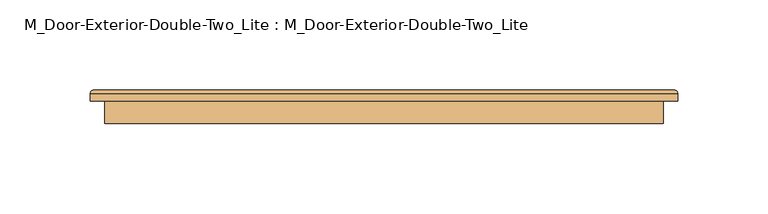
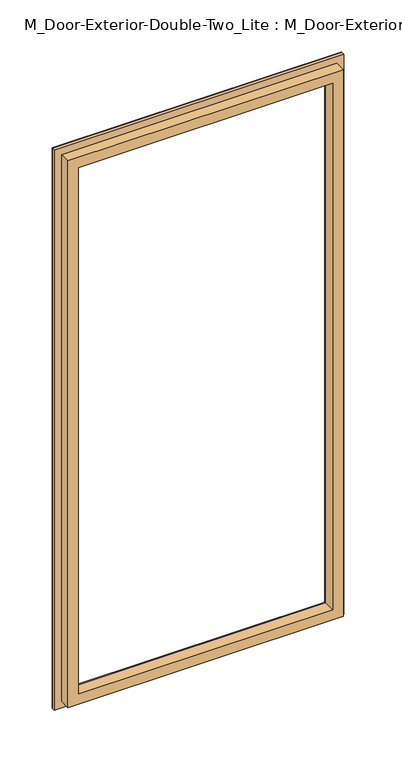
"""IFC4 building model written with IfcOpenShell, lengths in millimetres: door geometry, M_Door-Exterior-Double-Two_Lite : M_Door-Exterior-Double-Two_Lite."""

from ifc_helpers import new_model, si_unit, frame, origin, place, context, project, spatial, ellipse_curve, source, transform, mapped, element, save
from ifc_brep_helpers import plane_surface, cylinder_surface, advanced_brep


def m_door_exterior_double_two_lite_m_door_exterior_double_two_ddc6e1ea(model_context):
    return source(origin(), model_context, "Body", "AdvancedBrep", [
        advanced_brep(
        [(-459.6, 83.15, 900.0), (-459.6, 95.65, 900.0), (-459.6, 95.65, 250.0), (-459.6, 83.15, 250.0), (-447.6, 96.65, 888.0), (-447.6, 83.15, 888.0), (-447.6, 83.15, 262.0), (-447.6, 96.65, 262.0), (-452.6, 101.65, 893.0), (-452.6, 101.65, 257.0), (-467.6, 99.65, 908.0), (-465.6, 101.65, 906.0), (-465.6, 101.65, 244.0), (-467.6, 99.65, 242.0), (-467.6, 95.65, 908.0), (-467.6, 95.65, 242.0), (-150.0, 95.65, 250.0), (-150.0, 83.15, 250.0), (-162.0, 83.15, 262.0), (-162.0, 96.65, 262.0), (-157.0, 101.65, 257.0), (-144.0, 101.65, 244.0), (-142.0, 99.65, 242.0), (-142.0, 95.65, 242.0), (-150.0, 95.65, 900.0), (-150.0, 83.15, 900.0), (-162.0, 83.15, 888.0), (-162.0, 96.65, 888.0), (-157.0, 101.65, 893.0), (-144.0, 101.65, 906.0), (-142.0, 99.65, 908.0), (-142.0, 95.65, 908.0)],
        [
            (0, 1),
            (1, 2),
            (2, 3),
            (3, 0),
            (4, 5),
            (5, 6),
            (6, 7),
            (7, 4),
            (8, 4, ellipse_curve(frame((-452.6, 96.65, 893.0), z_axis=(-0.7071067811865475, 0.0, -0.7071067811865475), x_axis=(-0.7071067811865474, 0.0, 0.7071067811865476)), 7.0710678, 5.0)),
            (7, 9, ellipse_curve(frame((-452.6, 96.65, 257.0), z_axis=(-0.7071067811865475, 0.0, 0.7071067811865475), x_axis=(0.7071067811865474, 0.0, 0.7071067811865476)), 7.0710678, 5.0)),
            (9, 8),
            (10, 11, ellipse_curve(frame((-465.6, 99.65, 906.0), z_axis=(-0.7071067811865475, 0.0, -0.7071067811865475), x_axis=(-0.7071067811865474, 0.0, 0.7071067811865476)), 2.8284271, 2.0)),
            (11, 12),
            (12, 13, ellipse_curve(frame((-465.6, 99.65, 244.0), z_axis=(-0.7071067811865475, 0.0, 0.7071067811865475), x_axis=(0.7071067811865474, 0.0, 0.7071067811865476)), 2.8284271, 2.0)),
            (13, 10),
            (14, 10),
            (13, 15),
            (15, 14),
            (2, 16),
            (16, 17),
            (17, 3),
            (6, 18),
            (18, 19),
            (19, 7),
            (19, 20, ellipse_curve(frame((-157.0, 96.65, 257.0), z_axis=(-0.7071067811865475, 0.0, -0.7071067811865475), x_axis=(-0.7071067811865476, 0.0, 0.7071067811865474)), 7.0710678, 5.0)),
            (20, 9),
            (12, 21),
            (21, 22, ellipse_curve(frame((-144.0, 99.65, 244.0), z_axis=(-0.7071067811865475, 0.0, -0.7071067811865475), x_axis=(-0.7071067811865476, 0.0, 0.7071067811865474)), 2.8284271, 2.0)),
            (22, 13),
            (22, 23),
            (23, 15),
            (16, 24),
            (24, 25),
            (25, 17),
            (18, 26),
            (26, 27),
            (27, 19),
            (27, 28, ellipse_curve(frame((-157.0, 96.65, 893.0), z_axis=(0.7071067811865475, 0.0, -0.7071067811865475), x_axis=(-0.7071067811865474, 0.0, -0.7071067811865476)), 7.0710678, 5.0)),
            (28, 20),
            (21, 29),
            (29, 30, ellipse_curve(frame((-144.0, 99.65, 906.0), z_axis=(0.7071067811865475, 0.0, -0.7071067811865475), x_axis=(-0.7071067811865474, 0.0, -0.7071067811865476)), 2.8284271, 2.0)),
            (30, 22),
            (30, 31),
            (31, 23),
            (31, 14),
            (1, 24),
            (0, 25),
            (5, 26),
            (4, 27),
            (8, 28),
            (11, 29),
            (10, 30),
        ],
        [
            plane_surface(frame((-459.6, 95.65, 900.0), z_axis=(-1.0, 0.0, 0.0), x_axis=(0.0, 0.0, -1.0))),
            plane_surface(frame((-447.6, 83.15, 888.0), z_axis=(1.0, 0.0, 0.0), x_axis=(0.0, 0.0, -1.0))),
            cylinder_surface(frame((-452.6, 96.65, 900.0), z_axis=(0.0, 0.0, 1.0), x_axis=(-1.0, 0.0, 0.0)), 5.0),
            cylinder_surface(frame((-465.6, 99.65, 900.0), z_axis=(0.0, 0.0, 1.0), x_axis=(-1.0, 0.0, 0.0)), 2.0),
            plane_surface(frame((-467.6, 99.65, 908.0), z_axis=(-1.0, 0.0, 0.0), x_axis=(0.0, 0.0, -1.0))),
            plane_surface(frame((-459.6, 95.65, 250.0), z_axis=(0.0, 0.0, -1.0), x_axis=(1.0, 0.0, 0.0))),
            plane_surface(frame((-447.6, 83.15, 262.0), z_axis=(0.0, 0.0, 1.0), x_axis=(1.0, 0.0, 0.0))),
            cylinder_surface(frame((-459.6, 96.65, 257.0), z_axis=(-1.0, 0.0, 0.0), x_axis=(0.0, 0.0, -1.0)), 5.0),
            cylinder_surface(frame((-459.6, 99.65, 244.0), z_axis=(-1.0, 0.0, 0.0), x_axis=(0.0, 0.0, -1.0)), 2.0),
            plane_surface(frame((-467.6, 99.65, 242.0), z_axis=(0.0, 0.0, -1.0), x_axis=(1.0, 0.0, 0.0))),
            plane_surface(frame((-150.0, 95.65, 250.0), z_axis=(1.0, 0.0, 0.0), x_axis=(0.0, 0.0, 1.0))),
            plane_surface(frame((-162.0, 83.15, 262.0), z_axis=(-1.0, 0.0, 0.0), x_axis=(0.0, 0.0, 1.0))),
            cylinder_surface(frame((-157.0, 96.65, 250.0), z_axis=(0.0, 0.0, -1.0), x_axis=(1.0, 0.0, 0.0)), 5.0),
            cylinder_surface(frame((-144.0, 99.65, 250.0), z_axis=(0.0, 0.0, -1.0), x_axis=(1.0, 0.0, 0.0)), 2.0),
            plane_surface(frame((-142.0, 99.65, 242.0), z_axis=(1.0, 0.0, 0.0), x_axis=(0.0, 0.0, 1.0))),
            plane_surface(frame((-142.0, 95.65, 908.0), z_axis=(0.0, -1.0, 0.0), x_axis=(-1.0, 0.0, 0.0))),
            plane_surface(frame((-150.0, 95.65, 900.0), z_axis=(0.0, 0.0, 1.0), x_axis=(-1.0, 0.0, 0.0))),
            plane_surface(frame((-150.0, 83.15, 900.0), z_axis=(0.0, -1.0, 0.0), x_axis=(-1.0, 0.0, 0.0))),
            plane_surface(frame((-162.0, 83.15, 888.0), z_axis=(0.0, 0.0, -1.0), x_axis=(-1.0, 0.0, 0.0))),
            cylinder_surface(frame((-150.0, 96.65, 893.0), z_axis=(1.0, 0.0, 0.0), x_axis=(0.0, 0.0, 1.0)), 5.0),
            plane_surface(frame((-157.0, 101.65, 893.0), z_axis=(0.0, 1.0, 0.0), x_axis=(-1.0, 0.0, 0.0))),
            cylinder_surface(frame((-150.0, 99.65, 906.0), z_axis=(1.0, 0.0, 0.0), x_axis=(0.0, 0.0, 1.0)), 2.0),
            plane_surface(frame((-142.0, 99.65, 908.0), z_axis=(0.0, 0.0, 1.0), x_axis=(-1.0, 0.0, 0.0))),
        ],
        [
            (0, [[1, 2, 3, 4]]),
            (1, [[5, 6, 7, 8]]),
            (2, [[9, -8, 10, 11]]),
            (3, [[12, 13, 14, 15]]),
            (4, [[16, -15, 17, 18]]),
            (5, [[-3, 19, 20, 21]]),
            (6, [[-7, 22, 23, 24]]),
            (7, [[-10, -24, 25, 26]]),
            (8, [[-14, 27, 28, 29]]),
            (9, [[-17, -29, 30, 31]]),
            (10, [[-20, 32, 33, 34]]),
            (11, [[-23, 35, 36, 37]]),
            (12, [[-25, -37, 38, 39]]),
            (13, [[-28, 40, 41, 42]]),
            (14, [[-30, -42, 43, 44]]),
            (15, [[-31, -44, 45, -18], [46, -32, -19, -2]]),
            (16, [[-33, -46, -1, 47]]),
            (17, [[-21, -34, -47, -4], [48, -35, -22, -6]]),
            (18, [[-36, -48, -5, 49]]),
            (19, [[-38, -49, -9, 50]]),
            (20, [[51, -40, -27, -13], [-26, -39, -50, -11]]),
            (21, [[-41, -51, -12, 52]]),
            (22, [[-43, -52, -16, -45]]),
        ],
    ),
    ])


if __name__ == "__main__":
    model = new_model("IFC4")
    model_context = context("Model", 3, world=origin())
    ifc_project = project(units=[si_unit("LENGTHUNIT", "METRE", prefix="MILLI")], contexts=[model_context])
    site = spatial("IfcSite", under=ifc_project)
    building = spatial("IfcBuilding", under=site)
    placement = place(None, origin())
    m_door_exterior_double_two_lite_m_door_exterior_double_two_shape = m_door_exterior_double_two_lite_m_door_exterior_double_two_ddc6e1ea(model_context)
    element("IfcDoor", 1, ObjectType="M_Door-Exterior-Double-Two_Lite : M_Door-Exterior-Double-Two_Lite", at=placement, inside=building, context=model_context, shape_type="MappedRepresentation", body=[
        mapped(m_door_exterior_double_two_lite_m_door_exterior_double_two_shape, transform((0.0, 0.0, 0.0), x_axis=(1.0, 0.0, 0.0), y_axis=(0.0, 1.0, 0.0), z_axis=(0.0, 0.0, 1.0))),
    ])
    save(model, "model.ifc")

# Revit data of these elements
# Type "M_Door-Exterior-Double-Two_Lite : M_Door-Exterior-Double-Two_Lite"
#   Type Mark = "8"
#   Assembly Code = "B2030100"
#   Analytic Construction = "Metal frame, double glass door"
#   Top Rail = 0' - 4.72441"
#   Threshold Length [instance default] = 4' - 3.93701"
#   Threshold Offset [instance default] = 0' - 0.59055"
#   Thickness = 0' - 1.77165"
#   Thermal Resistance (R) = 1.3794 (h·ft²·°F)/BTU
#   Swing Angle [instance default] = 90.00°
#   Strike Height = 3' - 3.37008"
#   Stiles = 0' - 5.90551"
#   SinglePanelWidth = 2' - 0"
#   Rough Width [instance default] = 4' - 3.93701"
#   Rough Height [instance default] = 7' - 2.61417"
#   MFOpeningHeight [instance default] = 0' - 3.93701"
#   MFOpeningWidth [instance default] = 0' - 3.93701"
#   Lock Rail = 0' - 7.87402"
#   Inset Calculate [instance default] = 0' - 4.13386"
#   Masonry Inset [instance default] = 0' - 0.98425"
#   Height = 6' - 10.67717"
#   Width = 4' - 0"
#   Heat Transfer Coefficient (U) = 0.7250 BTU/(h·ft²·°F)
#   Glass Thickness = 0' - 0.7874"
#   Masonry Frame Depth = 0' - 5.90551"
#   Bottom Rail = 0' - 9.84252"
#   Threshold [instance default] = yes
#   Masonry Frame [instance default] = yes
#   Function = 1
#   Dry Wall Frame [instance default] = no
#   Threshold Material = Cherry
#   Panic Bar Material = Metal - Stainless Steel
#   Panel Material = Metal - Painted - Grey
#   Glass Stop Material = Metal - Painted - Grey
#   Frame Material = Metal - Painted - Grey
#   Exterior Pull Material = Metal - Stainless Steel
#   Visual Light Transmittance = 0
#   Solar Heat Gain Coefficient = 0
#   Wall Closure = (empty or 0)
# Element 1 (IfcDoor, "M_Door-Exterior-Double-Two_Lite : M_Door-Exterior-Double-Two_Lite")
#   Materials on its faces: "Metal - Painted - Grey", "Metal - Stainless Steel", "Glass", "Cherry"
# Materials
#   "Cherry": class "Wood", colour RGB 226 177 128, transparency 0, Description = "Prunus Serotina", Cost = 0
#   "Metal - Stainless Steel": class "Metal", colour RGB 247 247 247, transparency 0
#   "Metal - Painted - Grey": class "Paint", colour RGB 104 104 104, transparency 0, Cost = 0
#   "Glass": class "Glass", colour RGB 0 128 192, transparency 0.75, Description = "Soda Lime Glass", Cost = 0
